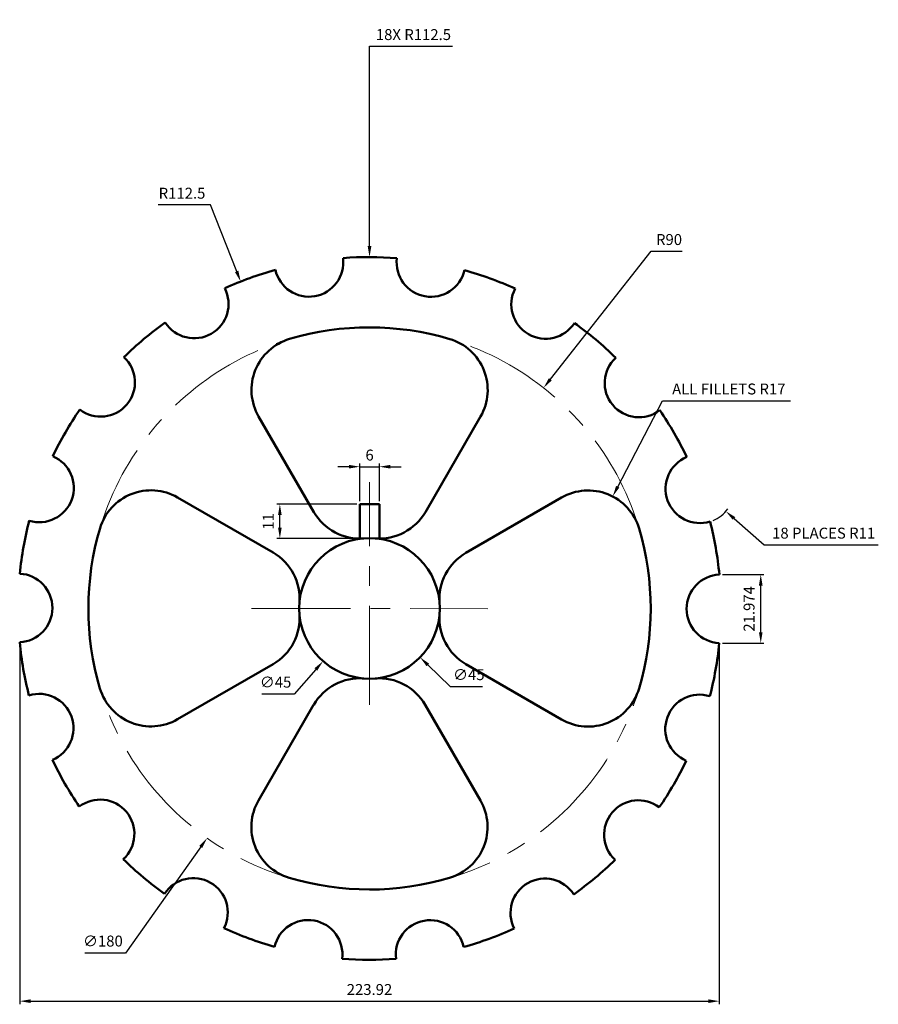
# Model space of a CAD drawing. Units: millimetres. Extents: x 3284 to 3559, y 1473 to 1788.
import ezdxf

# ---------------------------------------------------------------- set-up
doc = ezdxf.new("R2010")
doc.units = ezdxf.units.MM
doc.linetypes.add('CENTER', pattern=[50.8, 31.75, -6.35, 6.35, -6.35])
for name, color, linetype, lineweight in [('M-CNTR', 4, 'CENTER', 18), ('M-DIMS', 3, 'Continuous', 25), ('M-OUTL', 7, 'Continuous', 50)]:
    doc.layers.add(name, color=color, linetype=linetype, lineweight=lineweight)
doc.styles.get("Standard").update_dxf_attribs({"font": 'arial.ttf'})
doc.dimstyles.new('AM_ISO$0', dxfattribs={"dimtxt": 3.5, "dimasz": 3.5, "dimexe": 1, "dimexo": 1, "dimgap": 1.5, "dimtad": 1, "dimdsep": 46, "dimtxsty": 'Standard', "dimcen": 0, "dimclrd": 256, "dimclre": 256, "dimclrt": 2, "dimadec": 0, "dimazin": 2, "dimtp": 0.1, "dimtm": 0.1, "dimtfac": 0.71, "dimtdec": 3, "dimtmove": 0, "dimatfit": 3, "dimfxl": 1, "dimlwd": -1, "dimlwe": -1, "dimarcsym": 1})
doc.dimstyles.new('AM_ISO$3', dxfattribs={"dimtxt": 3.5, "dimasz": 3.5, "dimexe": 1, "dimexo": 1, "dimgap": 1.5, "dimtad": 1, "dimtoh": 1, "dimdsep": 46, "dimtxsty": 'Standard', "dimcen": 0, "dimclrd": 256, "dimclre": 256, "dimclrt": 2, "dimadec": 0, "dimazin": 2, "dimtp": 0.1, "dimtm": 0.1, "dimtfac": 0.71, "dimtdec": 3, "dimtofl": 0, "dimtmove": 0, "dimatfit": 0, "dimfxl": 1, "dimlwd": -1, "dimlwe": -1, "dimarcsym": 1})
doc.dimstyles.new('AM_ISO$4', dxfattribs={"dimtxt": 3.5, "dimasz": 3.5, "dimexe": 1, "dimexo": 1, "dimgap": 1.5, "dimtad": 1, "dimtoh": 1, "dimdsep": 46, "dimtxsty": 'Standard', "dimcen": 0, "dimclrd": 256, "dimclre": 256, "dimclrt": 2, "dimadec": 0, "dimazin": 2, "dimtp": 0.1, "dimtm": 0.1, "dimtfac": 0.71, "dimtdec": 3, "dimtofl": 0, "dimtmove": 0, "dimatfit": 0, "dimfxl": 1, "dimlwd": -1, "dimlwe": -1, "dimarcsym": 1})

# ---------------------------------------------------------------- blocks, each defined once
blk = doc.blocks.new('*U3')
blk.add_arc((5.76, 0), 11, 92.7308, 267.1263)
blk = doc.blocks.new('*U4')
at = {"layer": 'M-OUTL', "color": 0, "linetype": 'ByBlock', "lineweight": -2, "transparency": 16777216}
for p, rotation in [((3377.62, 1705.12), 99.99999999999984), ((3414.69, 1705.07), 79.9999999999999), ((3342.77, 1692.48), 119.9999999999999), ((3449.51, 1692.34), 59.99999999999999), ((3314.34, 1668.69), 139.9999999999998), ((3477.87, 1668.48), 39.99999999999999), ((3295.76, 1636.61), 159.9999999999998), ((3496.37, 1636.35), 19.99999999999995), ((3289.28, 1600.12), 180), ((3295.67, 1563.6), 199.9999999999996), ((3496.27, 1563.34), 339.9999999999995), ((3314.16, 1531.47), 219.9999999999995), ((3477.69, 1531.26), 319.9999999999996), ((3342.53, 1507.61), 239.9999999999996), ((3449.27, 1507.47), 299.9999999999996), ((3377.35, 1494.88), 259.9999999999996), ((3414.41, 1494.84), 279.9999999999995)]:
    blk.add_blockref('*U3', p, dxfattribs=dict(at, rotation=rotation))
blk.add_blockref('*U3', (3502.76, 1599.84), dxfattribs=at)
blk = doc.blocks.new('*D5')
at = {"layer": 'Defpoints', "color": 0, "transparency": 16777216}
for p in [(3473.85, 1635.83), (3466, 1620.75)]:
    blk.add_point(p, dxfattribs=at)
at = {"layer": 'M-DIMS', "color": 0, "linetype": 'ByBlock', "transparency": 16777216}
for p, q in [((3475.46, 1638.94), (3489.79, 1666.47)), ((3489.79, 1666.47), (3530.75, 1666.47))]:
    blk.add_line(p, q, dxfattribs=at)
at = {"layer": 'M-DIMS', "color": 0, "transparency": 16777216}
blk.add_solid([(3474.94, 1639.2), (3475.98, 1638.67), (3473.85, 1635.83)], dxfattribs=at)
at = {"layer": 'M-DIMS', "color": 0, "transparency": 16777216, "insert": (3511.02, 1669.78), "char_height": 3.5, "attachment_point": 5}
blk.add_mtext('ALL FILLETS R17', dxfattribs=at)
blk = doc.blocks.new('*U6')
for p, q in [((-25.31, 17.85), (5.29, 35.52)), ((-25.31, -17.86), (5.28, -35.52))]:
    blk.add_line(p, q)
for centre, radius, start, end in [((13.79, 20.8), 17, 16.5335, 120), ((-56.19, 0.02), 90, 343.427, 16.5335), ((-16.81, 3.13), 17, 120, 184.5083), ((-16.81, -3.13), 17, 175.413, 240), ((13.78, -20.8), 17, 240, 343.427)]:
    blk.add_arc(centre, radius, start, end)
blk = doc.blocks.new('*U7')
at = {"layer": 'M-OUTL', "color": 0, "linetype": 'ByBlock', "lineweight": -2, "transparency": 16777216}
for p, rotation in [((3396.04, 1656.16), 90.00000000000003), ((3339.83, 1600), 180), ((3395.99, 1543.79), 269.9999999999999)]:
    blk.add_blockref('*U6', p, dxfattribs=dict(at, rotation=rotation))
blk.add_blockref('*U6', (3452.2, 1599.95), dxfattribs=at)
blk = doc.blocks.new('*D8')
at = {"layer": 'Defpoints', "color": 0, "transparency": 16777216}
for p in [(3354.77, 1704.64), (3396.02, 1599.98)]:
    blk.add_point(p, dxfattribs=at)
at = {"layer": 'M-DIMS', "color": 0, "linetype": 'ByBlock', "transparency": 16777216}
for p, q in [((3345.1, 1729.19), (3328.41, 1729.19)), ((3353.49, 1707.9), (3345.1, 1729.19))]:
    blk.add_line(p, q, dxfattribs=at)
at = {"layer": 'M-DIMS', "color": 0, "transparency": 16777216}
blk.add_solid([(3354.03, 1708.11), (3352.94, 1707.68), (3354.77, 1704.64)], dxfattribs=at)
at = {"layer": 'M-DIMS', "color": 0, "transparency": 16777216, "insert": (3336, 1732.47), "char_height": 3.5, "attachment_point": 5}
blk.add_mtext('R112.5', dxfattribs=at)
blk = doc.blocks.new('*D9')
at = {"layer": 'Defpoints', "color": 0, "transparency": 16777216}
for p in [(3451.73, 1670.6), (3396.02, 1599.92)]:
    blk.add_point(p, dxfattribs=at)
at = {"layer": 'M-DIMS', "color": 0, "linetype": 'ByBlock', "transparency": 16777216}
for p, q in [((3453.89, 1673.35), (3486.21, 1714.36)), ((3486.21, 1714.36), (3496.06, 1714.36))]:
    blk.add_line(p, q, dxfattribs=at)
at = {"layer": 'M-DIMS', "color": 0, "transparency": 16777216}
blk.add_solid([(3453.43, 1673.71), (3454.35, 1672.99), (3451.73, 1670.6)], dxfattribs=at)
at = {"layer": 'M-DIMS', "color": 0, "transparency": 16777216, "insert": (3491.88, 1717.64), "char_height": 3.5, "attachment_point": 5}
blk.add_mtext('R90', dxfattribs=at)
blk = doc.blocks.new('*D10')
at = {"layer": 'Defpoints', "color": 0, "transparency": 16777216}
for p in [(3410.88, 1616.86), (3381.15, 1583.09)]:
    blk.add_point(p, dxfattribs=at)
at = {"layer": 'M-DIMS', "color": 0, "linetype": 'ByBlock', "transparency": 16777216}
for p, q in [((3378.84, 1580.46), (3371.87, 1572.55)), ((3371.87, 1572.55), (3361.53, 1572.55))]:
    blk.add_line(p, q, dxfattribs=at)
at = {"layer": 'M-DIMS', "color": 0, "transparency": 16777216}
blk.add_solid([(3378.4, 1580.84), (3379.28, 1580.07), (3381.15, 1583.09)], dxfattribs=at)
at = {"layer": 'M-DIMS', "color": 0, "transparency": 16777216, "insert": (3365.95, 1575.93), "char_height": 3.5, "attachment_point": 5}
blk.add_mtext('∅45', dxfattribs=at)
blk = doc.blocks.new('*D11')
at = {"layer": 'Defpoints', "color": 0, "transparency": 16777216}
for p in [(3367.31, 1633.35), (3392.91, 1633.35), (3392.91, 1622.35)]:
    blk.add_point(p, dxfattribs=at)
at = {"layer": 'M-DIMS', "color": 0, "linetype": 'ByBlock', "transparency": 16777216}
for p, q in [((3391.91, 1633.35), (3366.31, 1633.35)), ((3367.31, 1625.85), (3367.31, 1629.85)), ((3391.91, 1622.35), (3366.31, 1622.35))]:
    blk.add_line(p, q, dxfattribs=at)
at = {"layer": 'M-DIMS', "color": 0, "transparency": 16777216}
for points in [[(3366.73, 1629.85), (3367.9, 1629.85), (3367.31, 1633.35)], [(3366.73, 1625.85), (3367.9, 1625.85), (3367.31, 1622.35)]]:
    blk.add_solid(points, dxfattribs=at)
at = {"layer": 'M-DIMS', "color": 0, "transparency": 16777216, "insert": (3364.05, 1627.85), "char_height": 3.5, "attachment_point": 5, "rotation": 90}
blk.add_mtext('11', dxfattribs=at)
blk = doc.blocks.new('*D12')
at = {"layer": 'Defpoints', "color": 0, "transparency": 16777216}
for p in [(3399.18, 1645.35), (3392.91, 1633.35), (3399.18, 1633.35)]:
    blk.add_point(p, dxfattribs=at)
at = {"layer": 'M-DIMS', "color": 0, "linetype": 'ByBlock', "transparency": 16777216}
for p, q in [((3392.91, 1634.35), (3392.91, 1646.35)), ((3399.18, 1634.35), (3399.18, 1646.35)), ((3389.41, 1645.35), (3385.91, 1645.35)), ((3392.91, 1645.35), (3399.18, 1645.35)), ((3402.68, 1645.35), (3406.18, 1645.35))]:
    blk.add_line(p, q, dxfattribs=at)
at = {"layer": 'M-DIMS', "color": 0, "transparency": 16777216}
for points in [[(3389.41, 1645.94), (3389.41, 1644.77), (3392.91, 1645.35)], [(3402.68, 1645.94), (3402.68, 1644.77), (3399.18, 1645.35)]]:
    blk.add_solid(points, dxfattribs=at)
at = {"layer": 'M-DIMS', "color": 0, "transparency": 16777216, "insert": (3396.04, 1648.64), "char_height": 3.5, "attachment_point": 5}
blk.add_mtext('6', dxfattribs=at)
blk = doc.blocks.new('*D13')
at = {"layer": 'Defpoints', "color": 0, "transparency": 16777216}
for p in [(3501.78, 1638.32), (3510.06, 1631.08)]:
    blk.add_point(p, dxfattribs=at)
at = {"layer": 'M-DIMS', "color": 0, "linetype": 'ByBlock', "transparency": 16777216}
for p, q in [((3512.7, 1628.78), (3522.38, 1620.32)), ((3522.38, 1620.32), (3558.87, 1620.32))]:
    blk.add_line(p, q, dxfattribs=at)
blk.add_arc((3501.78, 1638.32), 11, 292.335, 324.0557, dxfattribs=at)
at = {"layer": 'M-DIMS', "color": 0, "transparency": 16777216}
blk.add_solid([(3513.08, 1629.22), (3512.31, 1628.34), (3510.06, 1631.08)], dxfattribs=at)
at = {"layer": 'M-DIMS', "color": 0, "transparency": 16777216, "insert": (3541.37, 1623.63), "char_height": 3.5, "attachment_point": 5}
blk.add_mtext('18 PLACES R11', dxfattribs=at)
blk = doc.blocks.new('*D14')
at = {"layer": 'Defpoints', "color": 0, "transparency": 16777216}
for p in [(3507.99, 1610.82), (3521.24, 1610.82), (3507.97, 1588.85)]:
    blk.add_point(p, dxfattribs=at)
at = {"layer": 'M-DIMS', "linetype": 'ByBlock', "transparency": 16777216}
for p, q in [((3508.99, 1610.82), (3522.24, 1610.82)), ((3521.24, 1592.35), (3521.24, 1607.32)), ((3508.97, 1588.85), (3522.24, 1588.85))]:
    blk.add_line(p, q, dxfattribs=at)
at = {"layer": 'M-DIMS', "transparency": 16777216}
for points in [[(3520.66, 1607.32), (3521.83, 1607.32), (3521.24, 1610.82)], [(3520.66, 1592.35), (3521.83, 1592.35), (3521.24, 1588.85)]]:
    blk.add_solid(points, dxfattribs=at)
at = {"layer": 'M-DIMS', "color": 2, "transparency": 16777216, "insert": (3517.96, 1599.84), "char_height": 3.5, "attachment_point": 5, "rotation": 90}
blk.add_mtext('21.974', dxfattribs=at)
blk = doc.blocks.new('*D15')
at = {"layer": 'Defpoints', "color": 0, "transparency": 16777216}
for p in [(3284.04, 1589.13), (3507.97, 1588.85), (3507.97, 1474.23)]:
    blk.add_point(p, dxfattribs=at)
at = {"layer": 'M-DIMS', "linetype": 'ByBlock', "transparency": 16777216}
for p, q in [((3284.04, 1588.13), (3284.04, 1473.23)), ((3507.97, 1587.85), (3507.97, 1473.23)), ((3287.54, 1474.23), (3504.47, 1474.23))]:
    blk.add_line(p, q, dxfattribs=at)
at = {"layer": 'M-DIMS', "transparency": 16777216}
for points in [[(3287.54, 1474.81), (3287.54, 1473.64), (3284.04, 1474.23)], [(3504.47, 1474.81), (3504.47, 1473.64), (3507.97, 1474.23)]]:
    blk.add_solid(points, dxfattribs=at)
at = {"layer": 'M-DIMS', "color": 2, "transparency": 16777216, "insert": (3396, 1477.51), "char_height": 3.5, "attachment_point": 5}
blk.add_mtext('223.92', dxfattribs=at)
blk = doc.blocks.new('*D16')
at = {"layer": 'Defpoints', "color": 0, "transparency": 16777216}
for p in [(3396.02, 1712.48), (3396.02, 1599.98)]:
    blk.add_point(p, dxfattribs=at)
at = {"layer": 'M-DIMS', "linetype": 'ByBlock', "transparency": 16777216}
for p, q in [((3396.02, 1715.98), (3396.02, 1779.98)), ((3396.02, 1779.98), (3422.61, 1779.98))]:
    blk.add_line(p, q, dxfattribs=at)
at = {"layer": 'M-DIMS', "transparency": 16777216}
blk.add_solid([(3396.6, 1715.98), (3395.43, 1715.98), (3396.02, 1712.48)], dxfattribs=at)
at = {"layer": 'M-DIMS', "color": 2, "transparency": 16777216, "insert": (3410.07, 1783.26), "char_height": 3.5, "attachment_point": 5}
blk.add_mtext('18X R112.5', dxfattribs=at)
blk = doc.blocks.new('*D17')
at = {"layer": 'Defpoints', "color": 0, "transparency": 16777216}
for p in [(3448.02, 1673.37), (3344.01, 1526.46)]:
    blk.add_point(p, dxfattribs=at)
at = {"layer": 'M-DIMS', "linetype": 'ByBlock', "transparency": 16777216}
for p, q in [((3341.99, 1523.61), (3317.95, 1489.64)), ((3317.95, 1489.64), (3304.92, 1489.64))]:
    blk.add_line(p, q, dxfattribs=at)
at = {"layer": 'M-DIMS', "transparency": 16777216}
blk.add_solid([(3341.52, 1523.94), (3342.47, 1523.27), (3344.01, 1526.46)], dxfattribs=at)
at = {"layer": 'M-DIMS', "color": 2, "transparency": 16777216, "insert": (3310.68, 1493.03), "char_height": 3.5, "attachment_point": 5}
blk.add_mtext('∅180', dxfattribs=at)
blk = doc.blocks.new('*D18')
at = {"layer": 'Defpoints', "color": 0, "transparency": 16777216}
for p in [(3379.86, 1615.63), (3412.18, 1584.32)]:
    blk.add_point(p, dxfattribs=at)
at = {"layer": 'M-DIMS', "linetype": 'ByBlock', "transparency": 16777216}
for p, q in [((3414.69, 1581.89), (3421.88, 1574.93)), ((3421.88, 1574.93), (3432.22, 1574.93))]:
    blk.add_line(p, q, dxfattribs=at)
at = {"layer": 'M-DIMS', "transparency": 16777216}
blk.add_solid([(3415.1, 1582.3), (3414.29, 1581.47), (3412.18, 1584.32)], dxfattribs=at)
at = {"layer": 'M-DIMS', "color": 2, "transparency": 16777216, "insert": (3427.8, 1578.31), "char_height": 3.5, "attachment_point": 5}
blk.add_mtext('∅45', dxfattribs=at)

msp = doc.modelspace()

# ---------------------------------------------------------------- linework, layer by layer
at = {"layer": 'M-CNTR'}
for p, q in [((3396.0174, 1569.0693), (3396.0174, 1640.3773)), ((3358.2176, 1599.9472), (3433.8486, 1599.8909))]:
    msp.add_line(p, q, dxfattribs=at)
msp.add_circle((3396.0174, 1599.9191), 89.9999, dxfattribs=at)
at = {"layer": 'M-OUTL'}
for p, q in [((3392.9125, 1622.3534), (3392.9125, 1633.3534)), ((3399.1763, 1633.3491), (3392.9125, 1633.3534)), ((3399.1763, 1622.3491), (3399.1763, 1633.3491))]:
    msp.add_line(p, q, dxfattribs=at)
msp.add_circle((3396.0174, 1599.9757), 22.5, dxfattribs=at)
for start, end in [(85.533053, 94.324077), (105.533053, 114.324077), (65.533053, 74.324077), (125.533053, 134.324077), (45.533053, 54.324077), (145.533053, 154.324077), (25.533053, 34.324077), (165.533053, 174.324077), (5.533053, 14.324077), (185.533053, 194.324077), (345.533053, 354.324077), (205.533053, 214.324077), (325.533053, 334.324077), (225.533053, 234.324077), (305.533053, 314.324077), (245.533053, 254.324077), (285.533053, 294.324077), (265.533053, 274.324077)]:
    msp.add_arc((3396.0174, 1599.9757), 112.5, start, end, dxfattribs=at)

# ---------------------------------------------------------------- block references
for name in ['*U4', '*U7']:
    msp.add_blockref(name, (0, 0), dxfattribs=at)

# ---------------------------------------------------------------- dimensions: what is measured, and where the dimension line sits
at = {"layer": 'M-DIMS'}
for center, mpoint, text, override, picture, middle in [((3396.0174, 1599.9757), (3396.017, 1712.4757), '18X <>', {"dimdec": 1, "dimlfac": 1, "dimrnd": 0, "dimzin": 0, "dimdsep": 46, "dimlunit": 2}, '*D16', (3410.0652, 1779.9757)), ((3465.9991, 1620.7497), (3473.846, 1635.8303), 'ALL FILLETS <>', {"dimpost": '', "dimclrd": 0, "dimclre": 0, "dimclrt": 0}, '*D5', (3511.0201, 1666.4748)), ((3501.7807, 1638.3211), (3510.0632, 1631.0823), '18 PLACES <>', {"dimclrd": 0, "dimclre": 0, "dimclrt": 0}, '*D13', (3541.3721, 1620.3203))]:
    dim = msp.add_radius_dim(center=center, mpoint=mpoint, text=text, dimstyle='AM_ISO$4', override=override, dxfattribs=at)
    dim.commit()
    dim.dimension.update_dxf_attribs({"geometry": picture, "text_midpoint": middle, "dimtype": 164})
for center, mpoint, override, picture, middle in [((3396.0174, 1599.9757), (3354.7686, 1704.6408), {"dimpost": '', "dimclrd": 0, "dimclre": 0, "dimclrt": 0}, '*D8', (3336.0023, 1729.1853)), ((3396.0174, 1599.9191), (3451.7265, 1670.6048), {"dimclrd": 0, "dimclre": 0, "dimclrt": 0}, '*D9', (3491.8842, 1714.3568))]:
    dim = msp.add_radius_dim(center=center, mpoint=mpoint, dimstyle='AM_ISO$4', override=override, dxfattribs=at)
    dim.commit()
    dim.dimension.update_dxf_attribs({"geometry": picture, "text_midpoint": middle, "dimtype": 164})
for p1, p2, dimstyle, override, picture, middle in [((3448.021, 1673.3739), (3344.0137, 1526.4642), 'AM_ISO$4', {"dimdec": 0, "dimlfac": 1, "dimrnd": 0, "dimzin": 0, "dimdsep": 46, "dimlunit": 2}, '*D17', (3310.6805, 1489.6423)), ((3410.8835, 1616.8649), (3381.1512, 1583.0864), 'AM_ISO$3', {"dimpost": '', "dimclrd": 0, "dimclre": 0, "dimclrt": 0}, '*D10', (3365.9494, 1572.546)), ((3379.8563, 1615.6304), (3412.1784, 1584.3209), 'AM_ISO$4', {"dimdec": 0, "dimlfac": 1, "dimrnd": 0, "dimzin": 0, "dimdsep": 46, "dimlunit": 2}, '*D18', (3427.799, 1574.9281))]:
    dim = msp.add_diameter_dim_2p(p1=p1, p2=p2, dimstyle=dimstyle, override=override, dxfattribs=at)
    dim.commit()
    dim.dimension.update_dxf_attribs({"geometry": picture, "text_midpoint": middle, "dimtype": 163})
for base, p1, p2, dimstyle, override, picture, middle in [((3399.1763, 1645.3534), (3392.9125, 1633.3534), (3399.1763, 1633.3534), 'AM_ISO$0', {"dimdec": 0, "dimclrd": 0, "dimclre": 0, "dimclrt": 0}, '*D12', (3396.0444, 1648.6404)), ((3507.9658, 1474.2257), (3284.0415, 1589.1284), (3507.9658, 1588.8492), 'AM_ISO$4', {"dimdec": 2, "dimlfac": 1, "dimrnd": 0, "dimzin": 0, "dimdsep": 46, "dimlunit": 2}, '*D15', (3396.0037, 1477.5139))]:
    dim = msp.add_linear_dim(base=base, p1=p1, p2=p2, dimstyle=dimstyle, override=override, dxfattribs=at)
    dim.commit()
    dim.dimension.update_dxf_attribs({"geometry": picture, "text_midpoint": middle})
for base, p1, p2, dimstyle, override, picture, middle in [((3367.3119, 1633.3534), (3392.9125, 1622.3534), (3392.9125, 1633.3534), 'AM_ISO$0', {"dimpost": '', "dimclrd": 0, "dimclre": 0, "dimclrt": 0}, '*D11', (3364.0547, 1627.8534)), ((3521.2432, 1610.8229), (3507.9658, 1588.8492), (3507.9932, 1610.8229), 'AM_ISO$4', {"dimdec": 3, "dimlfac": 1, "dimrnd": 0, "dimzin": 0, "dimdsep": 46, "dimlunit": 2}, '*D14', (3517.9562, 1599.8361))]:
    dim = msp.add_linear_dim(base=base, p1=p1, p2=p2, angle=90, dimstyle=dimstyle, override=override, dxfattribs=at)
    dim.commit()
    dim.dimension.update_dxf_attribs({"geometry": picture, "text_midpoint": middle})

doc.saveas('drawing.dxf')
